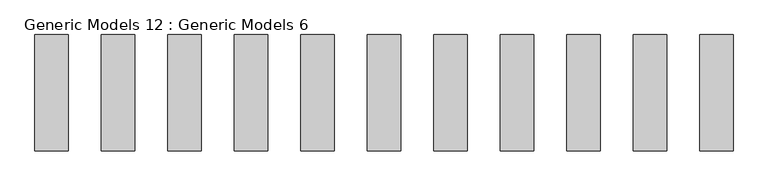
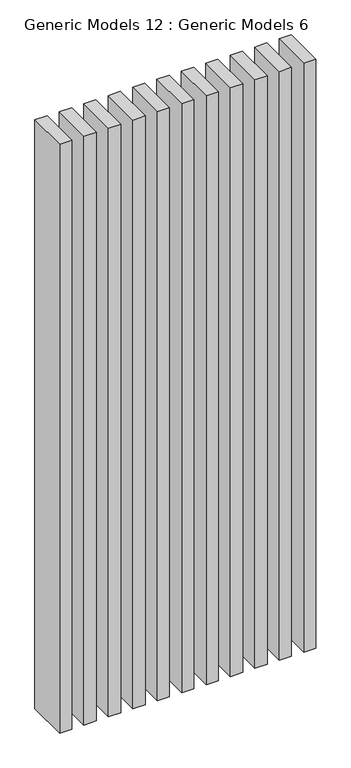
"""IFC4 building model written with IfcOpenShell, lengths in millimetres: proxy geometry, Generic Models 12 : Generic Models 6."""

from ifc_helpers import new_model, si_unit, frame, origin, place, context, project, spatial, polyline, outline, extrude, source, transform, mapped, element, save


def generic_models_12_generic_models_6_f1297f64(model_context):
    return source(origin(), model_context, "Body", "SweptSolid", [
        extrude(outline(polyline([(-7087.8263252, -11102.5719459), (-7138.6263252, -11102.5719459), (-7138.6263252, -10924.7719459), (-7087.8263252, -10924.7719459), (-7087.8263252, -11102.5719459)])), frame((0.0, 0.0, 9448.8), z_axis=(0.0, 0.0, 1.0), x_axis=(1.0, 0.0, 0.0)), (0.0, 0.0, 1.0), 2590.8),
        extrude(outline(polyline([(-6986.2263252, -11102.5719459), (-7037.0263252, -11102.5719459), (-7037.0263252, -10924.7719459), (-6986.2263252, -10924.7719459), (-6986.2263252, -11102.5719459)])), frame((0.0, 0.0, 9448.8), z_axis=(0.0, 0.0, 1.0), x_axis=(1.0, 0.0, 0.0)), (0.0, 0.0, 1.0), 2590.8),
        extrude(outline(polyline([(-6884.6263252, -11102.5719459), (-6935.4263252, -11102.5719459), (-6935.4263252, -10924.7719459), (-6884.6263252, -10924.7719459), (-6884.6263252, -11102.5719459)])), frame((0.0, 0.0, 9448.8), z_axis=(0.0, 0.0, 1.0), x_axis=(1.0, 0.0, 0.0)), (0.0, 0.0, 1.0), 2590.8),
        extrude(outline(polyline([(-6783.0263252, -11102.5719459), (-6833.8263252, -11102.5719459), (-6833.8263252, -10924.7719459), (-6783.0263252, -10924.7719459), (-6783.0263252, -11102.5719459)])), frame((0.0, 0.0, 9448.8), z_axis=(0.0, 0.0, 1.0), x_axis=(1.0, 0.0, 0.0)), (0.0, 0.0, 1.0), 2590.8),
        extrude(outline(polyline([(-6681.4263252, -11102.5719459), (-6732.2263252, -11102.5719459), (-6732.2263252, -10924.7719459), (-6681.4263252, -10924.7719459), (-6681.4263252, -11102.5719459)])), frame((0.0, 0.0, 9448.8), z_axis=(0.0, 0.0, 1.0), x_axis=(1.0, 0.0, 0.0)), (0.0, 0.0, 1.0), 2590.8),
        extrude(outline(polyline([(-6579.8263252, -11102.5719459), (-6630.6263252, -11102.5719459), (-6630.6263252, -10924.7719459), (-6579.8263252, -10924.7719459), (-6579.8263252, -11102.5719459)])), frame((0.0, 0.0, 9448.8), z_axis=(0.0, 0.0, 1.0), x_axis=(1.0, 0.0, 0.0)), (0.0, 0.0, 1.0), 2590.8),
        extrude(outline(polyline([(-6478.2263252, -11102.5719459), (-6529.0263252, -11102.5719459), (-6529.0263252, -10924.7719459), (-6478.2263252, -10924.7719459), (-6478.2263252, -11102.5719459)])), frame((0.0, 0.0, 9448.8), z_axis=(0.0, 0.0, 1.0), x_axis=(1.0, 0.0, 0.0)), (0.0, 0.0, 1.0), 2590.8),
        extrude(outline(polyline([(-6376.6263252, -11102.5719459), (-6427.4263252, -11102.5719459), (-6427.4263252, -10924.7719459), (-6376.6263252, -10924.7719459), (-6376.6263252, -11102.5719459)])), frame((0.0, 0.0, 9448.8), z_axis=(0.0, 0.0, 1.0), x_axis=(1.0, 0.0, 0.0)), (0.0, 0.0, 1.0), 2590.8),
        extrude(outline(polyline([(-6275.0263252, -11102.5719459), (-6325.8263252, -11102.5719459), (-6325.8263252, -10924.7719459), (-6275.0263252, -10924.7719459), (-6275.0263252, -11102.5719459)])), frame((0.0, 0.0, 9448.8), z_axis=(0.0, 0.0, 1.0), x_axis=(1.0, 0.0, 0.0)), (0.0, 0.0, 1.0), 2590.8),
        extrude(outline(polyline([(-6173.4263252, -11102.5719459), (-6224.2263252, -11102.5719459), (-6224.2263252, -10924.7719459), (-6173.4263252, -10924.7719459), (-6173.4263252, -11102.5719459)])), frame((0.0, 0.0, 9448.8), z_axis=(0.0, 0.0, 1.0), x_axis=(1.0, 0.0, 0.0)), (0.0, 0.0, 1.0), 2590.8),
        extrude(outline(polyline([(-6071.8263252, -11102.5719459), (-6122.6263252, -11102.5719459), (-6122.6263252, -10924.7719459), (-6071.8263252, -10924.7719459), (-6071.8263252, -11102.5719459)])), frame((0.0, 0.0, 9448.8), z_axis=(0.0, 0.0, 1.0), x_axis=(1.0, 0.0, 0.0)), (0.0, 0.0, 1.0), 2590.8),
    ])


if __name__ == "__main__":
    model = new_model("IFC4")
    model_context = context("Model", 3, world=origin())
    ifc_project = project(units=[si_unit("LENGTHUNIT", "METRE", prefix="MILLI")], contexts=[model_context])
    site = spatial("IfcSite", under=ifc_project)
    building = spatial("IfcBuilding", under=site)
    placement = place(None, origin())
    generic_models_12_generic_models_6_shape = generic_models_12_generic_models_6_f1297f64(model_context)
    element("IfcBuildingElementProxy", 1, Name="Generic Models 12 : Generic Models 6", ObjectType="Generic Models 12 : Generic Models 6", at=placement, inside=building, context=model_context, shape_type="MappedRepresentation", body=[
        mapped(generic_models_12_generic_models_6_shape, transform((0.0, 0.0, 0.0), x_axis=(1.0, 0.0, 0.0), y_axis=(0.0, 1.0, 0.0), z_axis=(0.0, 0.0, 1.0))),
    ])
    save(model, "model.ifc")

# Revit data of these elements
# Element 1 (IfcBuildingElementProxy, "Generic Models 12 : Generic Models 6")
#   Materials on its faces: "TEAK BROWN COLOUR"
# Materials
#   "TEAK BROWN COLOUR": class "Generic", colour RGB 120 120 120, transparency 0, Cost = 0
